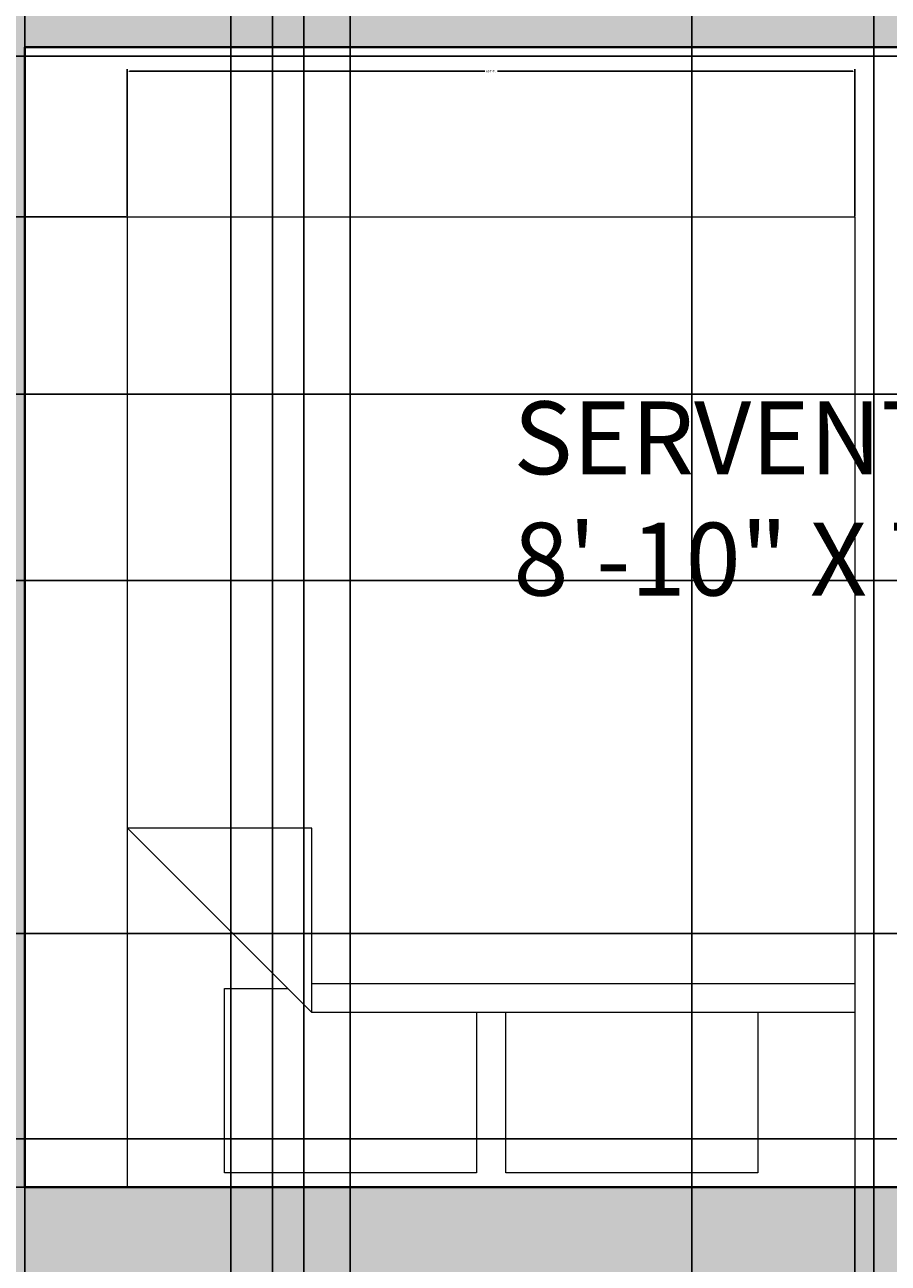
# Model space of a CAD drawing. Units: inches. Extents: x 818 to 1898, y 976 to 2364.
# Tile 52 of 96: x 1600 to 1671, y 1690 to 1792. Entities that reach past the tile are written whole.
import ezdxf

# ---------------------------------------------------------------- set-up
doc = ezdxf.new("R2010")
doc.units = ezdxf.units.IN
doc.header["$LTSCALE"] = 5
doc.header["$MEASUREMENT"] = 0
for name, color, linetype, lineweight in [('A-ANNO-DIMS', 2, 'Continuous', 18), ('A-AREA-IDEN', 7, 'Continuous', 18), ('A-FURN', 8, 'Continuous', 18), ('A-WALL', 7, 'Continuous', 40)]:
    doc.layers.add(name, color=color, linetype=linetype, lineweight=lineweight)
doc.layers.add('A-WALL-PATT', color=251, linetype='Continuous', lineweight=13, true_color=0x636466)
doc.styles.get("Standard").update_dxf_attribs({"font": 'arial.ttf'})
doc.dimstyles.get("Standard").update_dxf_attribs({"dimtxt": 0.18, "dimasz": 0.18, "dimexe": 0.18, "dimexo": 0.0625, "dimgap": 0.09, "dimtad": 0, "dimtih": 1, "dimtoh": 1, "dimdec": 4, "dimzin": 0, "dimdsep": 46, "dimtxsty": 'Standard', "dimcen": 0.09, "dimadec": 0, "dimazin": 0, "dimtfac": 1, "dimtdec": 4, "dimtofl": 0, "dimtmove": 0, "dimatfit": 3, "dimfxl": 1, "dimtolj": 1, "dimtzin": 0, "dimarcsym": 0})

# ---------------------------------------------------------------- blocks, each defined once
blk = doc.blocks.new('Bed - Queen')
for p, q in [((0, -80.00003), (0, 0)), ((0, 0), (59.99999, 0)), ((59.99999, 0), (59.99999, -80.00003)), ((7.99999, -1.2), (28.79998, -1.2)), ((7.99999, -14.4), (7.99999, -1.2)), ((28.79998, -1.2), (28.79998, -14.4)), ((31.19999, -1.2), (51.99999, -1.2)), ((31.19999, -14.4), (31.19999, -1.2)), ((51.99999, -1.2), (51.99999, -16.4)), ((0, -14.4), (44.8, -14.4)), ((59.99999, -29.6), (44.8, -14.4)), ((44.8, -14.4), (44.8, -29.6)), ((44.8, -16.8), (0, -16.8)), ((51.99999, -16.4), (46.79936, -16.4)), ((44.8, -29.6), (59.99999, -29.6)), ((59.99999, -80.00003), (0, -80.00003))]:
    blk.add_line(p, q)
blk = doc.blocks.new('*D46')
at = {"layer": 'A-ANNO-DIMS', "color": 0, "lineweight": -2, "ltscale": 5, "transparency": 16777216}
for p, q in [((1608.12, 1776.08), (1596, 1776.08)), ((1596.18, 1775.9), (1596.18, 1736.27)), ((1596.18, 1696.26), (1596.18, 1735.89)), ((1608.12, 1696.08), (1596, 1696.08))]:
    blk.add_line(p, q, dxfattribs=at)
at = {"layer": 'A-ANNO-DIMS', "color": 0, "ltscale": 5, "transparency": 16777216}
for points in [[(1596.15, 1775.9), (1596.21, 1775.9), (1596.18, 1776.08)], [(1596.15, 1696.26), (1596.21, 1696.26), (1596.18, 1696.08)]]:
    blk.add_solid(points, dxfattribs=at)
at = {"layer": 'Defpoints', "color": 0, "ltscale": 5, "transparency": 16777216}
for p in [(1608.18, 1776.08), (1596.18, 1696.08), (1608.18, 1696.08)]:
    blk.add_point(p, dxfattribs=at)
at = {"layer": 'A-ANNO-DIMS', "color": 0, "ltscale": 5, "transparency": 16777216, "insert": (1596.18, 1736.08), "char_height": 0.18, "attachment_point": 5}
blk.add_mtext('\\A1;QUEEN BED 80 TYP.', dxfattribs=at)
blk = doc.blocks.new('*D47')
at = {"layer": 'A-ANNO-DIMS', "color": 0, "lineweight": -2, "ltscale": 5, "transparency": 16777216}
for p, q in [((1608.18, 1776.14), (1608.18, 1788.26)), ((1608.36, 1788.08), (1637.66, 1788.08)), ((1668, 1788.08), (1638.71, 1788.08)), ((1668.18, 1776.14), (1668.18, 1788.26))]:
    blk.add_line(p, q, dxfattribs=at)
at = {"layer": 'A-ANNO-DIMS', "color": 0, "ltscale": 5, "transparency": 16777216}
for points in [[(1608.36, 1788.11), (1608.36, 1788.05), (1608.18, 1788.08)], [(1668, 1788.11), (1668, 1788.05), (1668.18, 1788.08)]]:
    blk.add_solid(points, dxfattribs=at)
at = {"layer": 'Defpoints', "color": 0, "ltscale": 5, "transparency": 16777216}
for p in [(1608.18, 1788.08), (1608.18, 1776.08), (1668.18, 1776.08)]:
    blk.add_point(p, dxfattribs=at)
at = {"layer": 'A-ANNO-DIMS', "color": 0, "ltscale": 5, "transparency": 16777216, "insert": (1638.18, 1788.08), "char_height": 0.18, "attachment_point": 5}
blk.add_mtext('\\A1;60 TYP.', dxfattribs=at)
blk = doc.blocks.new('*D85')
at = {"layer": 'A-ANNO-DIMS', "color": 0, "lineweight": -2, "ltscale": 5, "transparency": 16777216}
for p, q in [((1258.79, 2053.08), (1897.92, 2053.08)), ((1897.74, 2052.9), (1897.74, 1876.76)), ((1897.74, 1700.26), (1897.74, 1876.4)), ((1258.79, 1700.08), (1897.92, 1700.08))]:
    blk.add_line(p, q, dxfattribs=at)
at = {"layer": 'A-ANNO-DIMS', "color": 0, "ltscale": 5, "transparency": 16777216}
for points in [[(1897.71, 2052.9), (1897.77, 2052.9), (1897.74, 2053.08)], [(1897.71, 1700.26), (1897.77, 1700.26), (1897.74, 1700.08)]]:
    blk.add_solid(points, dxfattribs=at)
at = {"layer": 'Defpoints', "color": 0, "ltscale": 5, "transparency": 16777216}
for p in [(1258.73, 2053.08), (1897.74, 2053.08), (1258.73, 1700.08)]:
    blk.add_point(p, dxfattribs=at)
at = {"layer": 'A-ANNO-DIMS', "color": 0, "ltscale": 5, "transparency": 16777216, "insert": (1897.74, 1876.58), "char_height": 0.18, "attachment_point": 5}
blk.add_mtext('\\A1;353', dxfattribs=at)
blk = doc.blocks.new('*D102')
at = {"layer": 'A-ANNO-DIMS', "color": 0, "lineweight": -2, "ltscale": 5, "transparency": 16777216}
for p, q in [((1565.48, 1071.12), (1565.48, 2363.87)), ((1565.66, 2363.69), (1595.63, 2363.69)), ((1626.39, 2363.69), (1596.42, 2363.69)), ((1626.57, 1071.12), (1626.57, 2363.87))]:
    blk.add_line(p, q, dxfattribs=at)
at = {"layer": 'A-ANNO-DIMS', "color": 0, "ltscale": 5, "transparency": 16777216}
for points in [[(1565.66, 2363.72), (1565.66, 2363.66), (1565.48, 2363.69)], [(1626.39, 2363.72), (1626.39, 2363.66), (1626.57, 2363.69)]]:
    blk.add_solid(points, dxfattribs=at)
at = {"layer": 'Defpoints', "color": 0, "ltscale": 5, "transparency": 16777216}
for p in [(1626.57, 2363.69), (1565.48, 1071.06), (1626.57, 1071.06)]:
    blk.add_point(p, dxfattribs=at)
at = {"layer": 'A-ANNO-DIMS', "color": 0, "ltscale": 5, "transparency": 16777216, "insert": (1596.03, 2363.69), "char_height": 0.18, "attachment_point": 5}
blk.add_mtext('\\A1;61.09', dxfattribs=at)
blk = doc.blocks.new('*D103')
at = {"layer": 'A-ANNO-DIMS', "color": 0, "lineweight": -2, "ltscale": 5, "transparency": 16777216}
for p, q in [((1626.57, 1071.12), (1626.57, 2363.87)), ((1626.75, 2363.69), (1657.7, 2363.69)), ((1689.29, 2363.69), (1658.35, 2363.69)), ((1689.47, 1071.12), (1689.47, 2363.87))]:
    blk.add_line(p, q, dxfattribs=at)
at = {"layer": 'A-ANNO-DIMS', "color": 0, "ltscale": 5, "transparency": 16777216}
for points in [[(1626.75, 2363.72), (1626.75, 2363.66), (1626.57, 2363.69)], [(1689.29, 2363.72), (1689.29, 2363.66), (1689.47, 2363.69)]]:
    blk.add_solid(points, dxfattribs=at)
at = {"layer": 'Defpoints', "color": 0, "ltscale": 5, "transparency": 16777216}
for p in [(1689.47, 2363.69), (1626.57, 1071.06), (1689.47, 1071.06)]:
    blk.add_point(p, dxfattribs=at)
at = {"layer": 'A-ANNO-DIMS', "color": 0, "ltscale": 5, "transparency": 16777216, "insert": (1658.02, 2363.69), "char_height": 0.18, "attachment_point": 5}
blk.add_mtext('\\A1;62.9', dxfattribs=at)
blk = doc.blocks.new('*D119')
at = {"layer": 'A-ANNO-DIMS', "color": 0, "lineweight": -2, "ltscale": 5, "transparency": 16777216}
for p, q in [((1766.29, 1716.99), (818.03, 1716.99)), ((818.21, 1716.81), (818.21, 1672.43)), ((818.21, 1627.69), (818.21, 1672.06)), ((1766.29, 1627.51), (818.03, 1627.51))]:
    blk.add_line(p, q, dxfattribs=at)
at = {"layer": 'A-ANNO-DIMS', "color": 0, "ltscale": 5, "transparency": 16777216}
for points in [[(818.18, 1716.81), (818.24, 1716.81), (818.21, 1716.99)], [(818.18, 1627.69), (818.24, 1627.69), (818.21, 1627.51)]]:
    blk.add_solid(points, dxfattribs=at)
at = {"layer": 'Defpoints', "color": 0, "ltscale": 5, "transparency": 16777216}
for p in [(818.21, 1716.99), (1766.35, 1716.99), (1766.35, 1627.51)]:
    blk.add_point(p, dxfattribs=at)
at = {"layer": 'A-ANNO-DIMS', "color": 0, "ltscale": 5, "transparency": 16777216, "insert": (818.21, 1672.25), "char_height": 0.18, "attachment_point": 5}
blk.add_mtext('\\A1;89.48', dxfattribs=at)
blk = doc.blocks.new('*D120')
at = {"layer": 'A-ANNO-DIMS', "color": 0, "lineweight": -2, "ltscale": 5, "transparency": 16777216}
for p, q in [((1766.29, 1797.72), (818.03, 1797.72)), ((818.21, 1797.54), (818.21, 1757.53)), ((818.21, 1717.17), (818.21, 1757.17)), ((1766.29, 1716.99), (818.03, 1716.99))]:
    blk.add_line(p, q, dxfattribs=at)
at = {"layer": 'A-ANNO-DIMS', "color": 0, "ltscale": 5, "transparency": 16777216}
for points in [[(818.18, 1797.54), (818.24, 1797.54), (818.21, 1797.72)], [(818.18, 1717.17), (818.24, 1717.17), (818.21, 1716.99)]]:
    blk.add_solid(points, dxfattribs=at)
at = {"layer": 'Defpoints', "color": 0, "ltscale": 5, "transparency": 16777216}
for p in [(818.21, 1797.72), (1766.35, 1797.72), (1766.35, 1716.99)]:
    blk.add_point(p, dxfattribs=at)
at = {"layer": 'A-ANNO-DIMS', "color": 0, "ltscale": 5, "transparency": 16777216, "insert": (818.21, 1757.35), "char_height": 0.18, "attachment_point": 5}
blk.add_mtext('\\A1;80.73', dxfattribs=at)
blk = doc.blocks.new('*D173')
at = {"layer": 'A-ANNO-DIMS', "color": 0, "lineweight": -2, "ltscale": 5, "transparency": 16777216}
for p, q in [((1622.73, 1463.14), (1622.73, 2363.87)), ((1622.91, 2363.69), (1638.51, 2363.69)), ((1654.55, 2363.69), (1638.94, 2363.69)), ((1654.73, 1463.14), (1654.73, 2363.87))]:
    blk.add_line(p, q, dxfattribs=at)
at = {"layer": 'A-ANNO-DIMS', "color": 0, "ltscale": 5, "transparency": 16777216}
for points in [[(1622.91, 2363.72), (1622.91, 2363.66), (1622.73, 2363.69)], [(1654.55, 2363.72), (1654.55, 2363.66), (1654.73, 2363.69)]]:
    blk.add_solid(points, dxfattribs=at)
at = {"layer": 'Defpoints', "color": 0, "ltscale": 5, "transparency": 16777216}
for p in [(1654.73, 2363.69), (1622.73, 1463.08), (1654.73, 1463.08)]:
    blk.add_point(p, dxfattribs=at)
at = {"layer": 'A-ANNO-DIMS', "color": 0, "ltscale": 5, "transparency": 16777216, "insert": (1638.73, 2363.69), "char_height": 0.18, "attachment_point": 5}
blk.add_mtext('\\A1;32', dxfattribs=at)
blk = doc.blocks.new('*D174')
at = {"layer": 'A-ANNO-DIMS', "color": 0, "lineweight": -2, "ltscale": 5, "transparency": 16777216}
for p, q in [((1616.73, 1416.75), (1616.73, 2363.87)), ((1616.91, 2363.69), (1619.58, 2363.69)), ((1622.55, 2363.69), (1619.87, 2363.69)), ((1622.73, 1416.75), (1622.73, 2363.87))]:
    blk.add_line(p, q, dxfattribs=at)
at = {"layer": 'A-ANNO-DIMS', "color": 0, "ltscale": 5, "transparency": 16777216}
for points in [[(1616.91, 2363.72), (1616.91, 2363.66), (1616.73, 2363.69)], [(1622.55, 2363.72), (1622.55, 2363.66), (1622.73, 2363.69)]]:
    blk.add_solid(points, dxfattribs=at)
at = {"layer": 'Defpoints', "color": 0, "ltscale": 5, "transparency": 16777216}
for p in [(1622.73, 2363.69), (1616.73, 1416.69), (1622.73, 1416.69)]:
    blk.add_point(p, dxfattribs=at)
at = {"layer": 'A-ANNO-DIMS', "color": 0, "ltscale": 5, "transparency": 16777216, "insert": (1619.73, 2363.69), "char_height": 0.18, "attachment_point": 5}
blk.add_mtext('\\A1;6', dxfattribs=at)
blk = doc.blocks.new('*D175')
at = {"layer": 'A-ANNO-DIMS', "color": 0, "lineweight": -2, "ltscale": 5, "transparency": 16777216}
for p, q in [((1559.73, 1647.64), (1559.73, 2363.87)), ((1559.91, 2363.69), (1614.45, 2363.69)), ((1669.55, 2363.69), (1615.01, 2363.69)), ((1669.73, 1647.64), (1669.73, 2363.87))]:
    blk.add_line(p, q, dxfattribs=at)
at = {"layer": 'A-ANNO-DIMS', "color": 0, "ltscale": 5, "transparency": 16777216}
for points in [[(1559.91, 2363.72), (1559.91, 2363.66), (1559.73, 2363.69)], [(1669.55, 2363.72), (1669.55, 2363.66), (1669.73, 2363.69)]]:
    blk.add_solid(points, dxfattribs=at)
at = {"layer": 'Defpoints', "color": 0, "ltscale": 5, "transparency": 16777216}
for p in [(1669.73, 2363.69), (1559.73, 1647.58), (1669.73, 1647.58)]:
    blk.add_point(p, dxfattribs=at)
at = {"layer": 'A-ANNO-DIMS', "color": 0, "ltscale": 5, "transparency": 16777216, "insert": (1614.73, 2363.69), "char_height": 0.18, "attachment_point": 5}
blk.add_mtext('\\A1;110', dxfattribs=at)
blk = doc.blocks.new('*D221')
at = {"layer": 'A-ANNO-DIMS', "color": 0, "lineweight": -2, "ltscale": 5, "transparency": 16777216}
for p, q in [((1668.18, 1696.02), (1668.18, 975.66)), ((1705.73, 1696.02), (1705.73, 975.66)), ((1668.36, 975.84), (1686.56, 975.84)), ((1705.55, 975.84), (1687.35, 975.84))]:
    blk.add_line(p, q, dxfattribs=at)
at = {"layer": 'A-ANNO-DIMS', "color": 0, "ltscale": 5, "transparency": 16777216}
for points in [[(1668.36, 975.87), (1668.36, 975.81), (1668.18, 975.84)], [(1705.55, 975.87), (1705.55, 975.81), (1705.73, 975.84)]]:
    blk.add_solid(points, dxfattribs=at)
at = {"layer": 'Defpoints', "color": 0, "ltscale": 5, "transparency": 16777216}
for p in [(1668.18, 1696.08), (1705.73, 1696.08), (1705.73, 975.84)]:
    blk.add_point(p, dxfattribs=at)
at = {"layer": 'A-ANNO-DIMS', "color": 0, "ltscale": 5, "transparency": 16777216, "insert": (1686.95, 975.84), "char_height": 0.18, "attachment_point": 5}
blk.add_mtext('\\A1;37.54', dxfattribs=at)
blk = doc.blocks.new('*D229')
at = {"layer": 'A-ANNO-DIMS', "color": 0, "lineweight": -2, "ltscale": 5, "transparency": 16777216}
for p, q in [((1599.73, 2044.02), (1599.73, 975.66)), ((1620.14, 2036.06), (1620.14, 975.66)), ((1599.91, 975.84), (1609.47, 975.84)), ((1619.96, 975.84), (1610.4, 975.84))]:
    blk.add_line(p, q, dxfattribs=at)
at = {"layer": 'A-ANNO-DIMS', "color": 0, "ltscale": 5, "transparency": 16777216}
for points in [[(1599.91, 975.87), (1599.91, 975.81), (1599.73, 975.84)], [(1619.96, 975.87), (1619.96, 975.81), (1620.14, 975.84)]]:
    blk.add_solid(points, dxfattribs=at)
at = {"layer": 'Defpoints', "color": 0, "ltscale": 5, "transparency": 16777216}
for p in [(1599.73, 2044.08), (1620.14, 2036.12), (1620.14, 975.84)]:
    blk.add_point(p, dxfattribs=at)
at = {"layer": 'A-ANNO-DIMS', "color": 0, "ltscale": 5, "transparency": 16777216, "insert": (1609.93, 975.84), "char_height": 0.18, "attachment_point": 5}
blk.add_mtext('\\A1;20.416', dxfattribs=at)
blk = doc.blocks.new('*D280')
at = {"layer": 'A-ANNO-DIMS', "color": 0, "lineweight": -2, "ltscale": 5, "transparency": 16777216}
for p, q in [((1398.73, 1789.31), (1897.92, 1789.31)), ((1897.74, 1789.13), (1897.74, 1767.89)), ((1897.74, 1746.29), (1897.74, 1767.53)), ((1397.41, 1746.11), (1897.92, 1746.11))]:
    blk.add_line(p, q, dxfattribs=at)
at = {"layer": 'A-ANNO-DIMS', "color": 0, "ltscale": 5, "transparency": 16777216}
for points in [[(1897.71, 1789.13), (1897.77, 1789.13), (1897.74, 1789.31)], [(1897.71, 1746.29), (1897.77, 1746.29), (1897.74, 1746.11)]]:
    blk.add_solid(points, dxfattribs=at)
at = {"layer": 'Defpoints', "color": 0, "ltscale": 5, "transparency": 16777216}
for p in [(1398.67, 1789.31), (1897.74, 1789.31), (1397.35, 1746.11)]:
    blk.add_point(p, dxfattribs=at)
at = {"layer": 'A-ANNO-DIMS', "color": 0, "ltscale": 5, "transparency": 16777216, "insert": (1897.74, 1767.71), "char_height": 0.18, "attachment_point": 5}
blk.add_mtext('\\A1;43.19', dxfattribs=at)
blk = doc.blocks.new('*D282')
at = {"layer": 'A-ANNO-DIMS', "color": 0, "lineweight": -2, "ltscale": 5, "transparency": 16777216}
for p, q in [((1422.08, 2081.19), (1897.92, 2081.19)), ((1897.74, 2081.01), (1897.74, 1884.32)), ((1897.74, 1687.26), (1897.74, 1883.95)), ((1463.79, 1687.08), (1897.92, 1687.08))]:
    blk.add_line(p, q, dxfattribs=at)
at = {"layer": 'A-ANNO-DIMS', "color": 0, "ltscale": 5, "transparency": 16777216}
for points in [[(1897.71, 2081.01), (1897.77, 2081.01), (1897.74, 2081.19)], [(1897.71, 1687.26), (1897.77, 1687.26), (1897.74, 1687.08)]]:
    blk.add_solid(points, dxfattribs=at)
at = {"layer": 'Defpoints', "color": 0, "ltscale": 5, "transparency": 16777216}
for p in [(1422.02, 2081.19), (1897.74, 2081.19), (1463.73, 1687.08)]:
    blk.add_point(p, dxfattribs=at)
at = {"layer": 'A-ANNO-DIMS', "color": 0, "ltscale": 5, "transparency": 16777216, "insert": (1897.74, 1884.13), "char_height": 0.18, "attachment_point": 5}
blk.add_mtext('\\A1;394.1', dxfattribs=at)
blk = doc.blocks.new('*D284')
at = {"layer": 'A-ANNO-DIMS', "color": 0, "lineweight": -2, "ltscale": 5, "transparency": 16777216}
for p, q in [((1351.66, 1761.45), (1897.92, 1761.45)), ((1897.74, 1761.27), (1897.74, 1728.95)), ((1897.74, 1696.26), (1897.74, 1728.58)), ((1267.79, 1696.08), (1897.92, 1696.08))]:
    blk.add_line(p, q, dxfattribs=at)
at = {"layer": 'A-ANNO-DIMS', "color": 0, "ltscale": 5, "transparency": 16777216}
for points in [[(1897.71, 1761.27), (1897.77, 1761.27), (1897.74, 1761.45)], [(1897.71, 1696.26), (1897.77, 1696.26), (1897.74, 1696.08)]]:
    blk.add_solid(points, dxfattribs=at)
at = {"layer": 'Defpoints', "color": 0, "ltscale": 5, "transparency": 16777216}
for p in [(1351.6, 1761.45), (1267.73, 1696.08), (1897.74, 1696.08)]:
    blk.add_point(p, dxfattribs=at)
at = {"layer": 'A-ANNO-DIMS', "color": 0, "ltscale": 5, "transparency": 16777216, "insert": (1897.74, 1728.76), "char_height": 0.18, "attachment_point": 5}
blk.add_mtext('\\A1;65.37', dxfattribs=at)

msp = doc.modelspace()

# ---------------------------------------------------------------- hatches: boundary and pattern name
at = {"layer": 'A-WALL-PATT', "ltscale": 5}
h = msp.add_hatch(color=256, dxfattribs=at)
h.dxf.hatch_style = 1
h.paths.add_polyline_path([(1267.7251, 1928.9218), (1258.7251, 1928.9218), (1258.7251, 1913.6401), (1250.3029, 1913.6401), (1250.3029, 1878.3919), (1258.7251, 1878.3919), (1258.7251, 1862.9652), (1267.7251, 1862.9652)])
h.paths.add_polyline_path([(1267.7251, 1814.9652), (1258.7251, 1814.9652), (1258.7251, 1755.3321), (1267.7251, 1755.3321)])
h.paths.add_polyline_path([(1463.7251, 1696.0782), (1267.7251, 1696.0782), (1267.7251, 1707.3321), (1258.7251, 1707.3321), (1258.7251, 1700.0782), (1251.9333, 1700.0782), (1251.9333, 1687.0782), (1463.7251, 1687.0782)])
h.paths.add_polyline_path([(1714.7252, 1717.3178), (1705.7251, 1717.3178), (1705.7251, 1696.0782), (1599.7251, 1696.0782), (1599.7251, 1790.0782), (1705.7251, 1790.0782), (1705.7251, 1785.6125), (1714.7252, 1785.6125), (1714.7252, 1827.2125), (1705.7251, 1827.2125), (1705.7251, 1802.0782), (1599.7251, 1802.0782), (1599.7251, 1867.0782), (1705.7251, 1867.0782), (1705.7251, 1857.2125), (1714.7252, 1857.2125), (1714.7252, 1930.0316), (1741.8409, 1930.0316), (1741.8409, 1935.0316), (1714.7252, 1935.0316), (1714.7252, 1957.0338), (1741.8409, 1957.0338), (1741.8409, 1962.0338), (1714.7252, 1962.0338), (1705.7251, 1962.0338), (1705.7251, 1948.0782), (1599.7251, 1948.0782), (1599.7251, 1981.0782), (1590.7252, 1981.0782), (1590.7252, 1941.0782), (1620.7252, 1941.0782), (1705.7251, 1941.0782), (1705.7251, 1876.0782), (1599.7251, 1876.0782), (1599.7251, 1911.0782), (1590.7252, 1911.0782), (1590.7252, 1876.0782), (1429.2252, 1876.0782), (1429.2252, 1867.0782), (1511.7252, 1867.0782), (1528.593, 1867.0782), (1595.7252, 1867.0782), (1595.7252, 1773.0782), (1520.7252, 1773.0782), (1520.7252, 1837.5823), (1532.593, 1837.5823), (1532.593, 1867.0782), (1528.593, 1867.0782), (1528.593, 1841.5823), (1511.7252, 1841.5823), (1511.7252, 1744.9714), (1520.7252, 1744.9714), (1520.7252, 1761.0782), (1595.7252, 1761.0782), (1595.7252, 1696.0782), (1520.7252, 1696.0782), (1520.7252, 1716.0454), (1511.7252, 1716.0454), (1511.7252, 1696.0782), (1511.7252, 1687.0782), (1714.7252, 1687.0782)])
h.paths.add_polyline_path([(1714.7252, 2053.0782), (1714.7252, 2081.1881), (1709.7252, 2081.1881), (1709.7252, 2053.0782), (1681.6446, 2053.0782), (1681.6446, 2081.1881), (1676.6446, 2081.1881), (1676.6446, 2053.0782), (1538.5155, 2053.0782), (1538.5155, 2044.0782), (1590.7252, 2044.0782), (1590.7252, 2011.0782), (1599.7251, 2011.0782), (1599.7251, 2044.0782), (1705.7251, 2044.0782), (1705.7251, 2014.5114), (1714.7252, 2014.5114)])
h.paths.add_polyline_path([(1485.1216, 2053.0782), (1422.02, 2053.0782), (1422.02, 2081.1881), (1413.02, 2081.1881), (1413.02, 2053.0782), (1399.6356, 2053.0782), (1399.6356, 2081.1881), (1390.6356, 2081.1881), (1390.6356, 2053.0782), (1388.0315, 2053.0782), (1388.0315, 2044.0782), (1416.2743, 2044.0782), (1485.1216, 2044.0782)])
h.paths.add_polyline_path([(1330.305, 2053.0782), (1258.7251, 2053.0782), (1258.7251, 2019.2871), (1267.7251, 2019.2871), (1267.7251, 2044.0782), (1330.305, 2044.0782)])
h.paths.add_polyline_path([(1258.7251, 2053.0782), (1214.6577, 2053.0782), (1214.6577, 2044.0782), (1258.7251, 2044.0782)])
h.paths.add_polyline_path([(1214.6577, 2053.0782), (1180.349, 2053.0782), (1180.349, 2044.0782), (1214.6577, 2044.0782)])
h.paths.add_polyline_path([(1714.7252, 1639.5782), (1741.8409, 1639.5782), (1741.8409, 1643.5782), (1714.7252, 1643.5782), (1714.7252, 1649.9029), (1705.7251, 1649.9029), (1705.7251, 1600.0782), (1477.7252, 1600.0782), (1477.7252, 1591.0782), (1520.7252, 1591.0782), (1616.7251, 1591.0782), (1616.7251, 1416.6857), (1622.7251, 1416.6857), (1622.7251, 1463.0782), (1624.7252, 1463.0782), (1624.7252, 1467.0782), (1622.7251, 1467.0782), (1622.7251, 1591.0782), (1705.7251, 1591.0782), (1705.7251, 1545.0782), (1714.7252, 1545.0782), (1741.8409, 1545.0782), (1741.8409, 1549.0782), (1714.7252, 1549.0782), (1714.7252, 1593.9175), (1737.8409, 1593.9175), (1737.8409, 1597.9175), (1714.7252, 1597.9175)])
h.paths.add_polyline_path([(1674.9024, 2060.7419), (1714.7045, 2060.7419), (1714.7045, 2073.1061), (1674.9024, 2073.1061)], flags=25)
h.paths.add_polyline_path([(1394.5468, 2061.6618), (1422.2344, 2061.6618), (1422.2344, 2074.0261), (1394.5468, 2074.0261)], flags=24)

# ---------------------------------------------------------------- linework, layer by layer
at = {"layer": 'A-WALL'}
for p, q in [((1599.7251, 1790.0782), (1705.7251, 1790.0782)), ((1599.7251, 1790.0782), (1599.7251, 1696.0782)), ((1599.7251, 1696.0782), (1705.7251, 1696.0782))]:
    msp.add_line(p, q, dxfattribs=at)

# ---------------------------------------------------------------- block references
at = {"layer": 'A-FURN', "rotation": 180}
msp.add_blockref('Bed - Queen', (1668.1841, 1696.0782), dxfattribs=at)

# ---------------------------------------------------------------- texts
at = {"layer": 'A-AREA-IDEN', "ltscale": 5, "insert": (1640.016, 1760.8611), "char_height": 6, "attachment_point": 1}
msp.add_mtext_dynamic_manual_height_columns('SERVENT ROON\\P8\'-10" X 7\'-10"', width=118.992422, gutter_width=1, heights=[0], dxfattribs=at)

# ---------------------------------------------------------------- dimensions: what is measured, and where the dimension line sits
at = {"layer": 'A-ANNO-DIMS', "ltscale": 5}
for base, p1, p2, override, picture, middle in [((1669.7251, 2363.6929), (1559.7251, 1647.5782), (1669.7251, 1647.5782), {"dimdec": 0, "dimlfac": 1, "dimrnd": 0, "dimzin": 0, "dimdsep": 46, "dimlunit": 2}, '*D175', (1614.7251, 2363.6929)), ((1626.5748, 2363.6929), (1565.4835, 1071.0552), (1626.5748, 1071.0552), {"dimdec": 2, "dimlfac": 1, "dimrnd": 0, "dimzin": 0, "dimdsep": 46, "dimlunit": 2}, '*D102', (1596.0291, 2363.6929)), ((1622.7251, 2363.6929), (1616.7251, 1416.6857), (1622.7251, 1416.6857), {"dimdec": 0, "dimlfac": 1, "dimrnd": 0, "dimzin": 0, "dimdsep": 46, "dimlunit": 2}, '*D174', (1619.7251, 2363.6929)), ((1654.7251, 2363.6929), (1622.7251, 1463.0782), (1654.7251, 1463.0782), {"dimdec": 0, "dimlfac": 1, "dimrnd": 0, "dimzin": 0, "dimdsep": 46, "dimlunit": 2}, '*D173', (1638.7251, 2363.6929)), ((1689.4714, 2363.6929), (1626.5748, 1071.0552), (1689.4714, 1071.0552), {"dimdec": 1, "dimlfac": 1, "dimrnd": 0, "dimzin": 0, "dimdsep": 46, "dimlunit": 2}, '*D103', (1658.0231, 2363.6929)), ((1620.14159, 975.84326), (1599.72515, 2044.07824), (1620.14159, 2036.1182), {"dimdec": 3, "dimlfac": 1, "dimrnd": 0, "dimzin": 0, "dimdsep": 46, "dimlunit": 2}, '*D229', (1609.93337, 975.84326)), ((1705.7251, 975.8433), (1668.1841, 1696.0782), (1705.7251, 1696.0782), {"dimdec": 2, "dimlfac": 1, "dimrnd": 0, "dimzin": 0, "dimdsep": 46, "dimlunit": 2}, '*D221', (1686.9546, 975.8433))]:
    dim = msp.add_linear_dim(base=base, p1=p1, p2=p2, dimstyle='Standard', override=override, dxfattribs=at)
    dim.commit()
    dim.dimension.update_dxf_attribs({"geometry": picture, "text_midpoint": middle})
for base, p1, p2, override, picture, middle in [((1897.736, 2081.1881), (1463.7251, 1687.0782), (1422.02, 2081.1881), {"dimdec": 1, "dimlfac": 1, "dimrnd": 0, "dimzin": 0, "dimdsep": 46, "dimlunit": 2}, '*D282', (1897.736, 1884.1332)), ((1897.736, 2053.0782), (1258.7251, 1700.0782), (1258.7251, 2053.0782), {"dimdec": 0, "dimlfac": 1, "dimrnd": 0, "dimzin": 0, "dimdsep": 46, "dimlunit": 2}, '*D85', (1897.736, 1876.5782)), ((818.2059, 1797.7165), (1766.3524, 1716.9866), (1766.3524, 1797.7165), {"dimdec": 2, "dimlfac": 1, "dimrnd": 0, "dimzin": 0, "dimdsep": 46, "dimlunit": 2}, '*D120', (818.2059, 1757.3516)), ((1897.736, 1789.3057), (1397.3459, 1746.1142), (1398.6717, 1789.3057), {"dimdec": 2, "dimlfac": 1, "dimrnd": 0, "dimzin": 0, "dimdsep": 46, "dimlunit": 2}, '*D280', (1897.736, 1767.71)), ((1897.736, 1696.0782), (1351.5985, 1761.449), (1267.7251, 1696.0782), {"dimdec": 2, "dimlfac": 1, "dimrnd": 0, "dimzin": 0, "dimdsep": 46, "dimlunit": 2}, '*D284', (1897.736, 1728.7636)), ((818.2059, 1716.9866), (1766.3524, 1627.5052), (1766.3524, 1716.9866), {"dimdec": 2, "dimlfac": 1, "dimrnd": 0, "dimzin": 0, "dimdsep": 46, "dimlunit": 2}, '*D119', (818.2059, 1672.2459))]:
    dim = msp.add_linear_dim(base=base, p1=p1, p2=p2, angle=90, dimstyle='Standard', override=override, dxfattribs=at)
    dim.commit()
    dim.dimension.update_dxf_attribs({"geometry": picture, "text_midpoint": middle})
for base, p1, p2, angle, text, picture, middle in [((1608.1842, 1788.0783), (1668.1841, 1776.0783), (1608.1842, 1776.0783), 180, '<> TYP.', '*D47', (1638.1841, 1788.0783)), ((1596.1841, 1696.0782), (1608.1842, 1776.0783), (1608.1842, 1696.0782), 270, 'QUEEN BED <> TYP.', '*D46', (1596.1841, 1736.0783))]:
    dim = msp.add_linear_dim(base=base, p1=p1, p2=p2, angle=angle, text=text, dimstyle='Standard', override={"dimdec": 0, "dimlfac": 1, "dimrnd": 0, "dimzin": 0, "dimdsep": 46, "dimlunit": 2}, dxfattribs=at)
    dim.commit()
    dim.dimension.update_dxf_attribs({"geometry": picture, "text_midpoint": middle})

doc.saveas('drawing.dxf')
